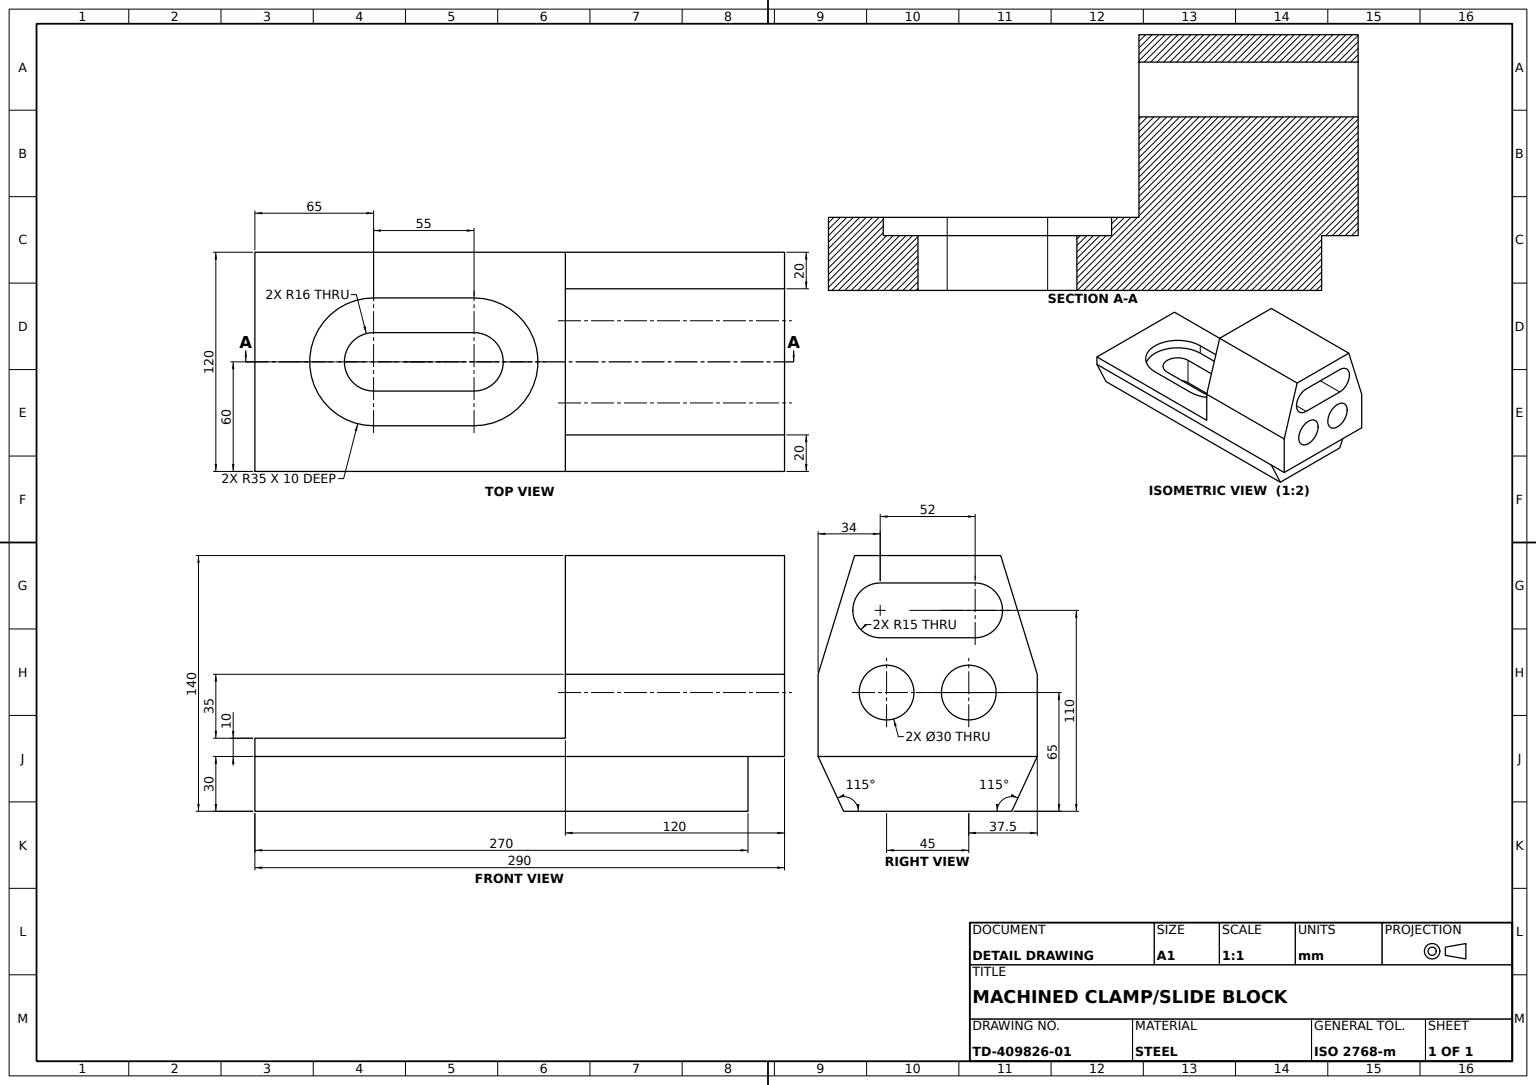
SolidWorks part; units mm, degrees
material "Plain Carbon Steel"
ref_plane "Front Plane" through (0, 0, 0) normal (0, 0, 1) x (1, 0, 0)
ref_plane "Top Plane" through (0, 0, 0) normal (0, 1, 0) x (1, 0, 0)
ref_plane "Right Plane" through (0, 0, 0) normal (1, 0, 0) x (0, 0, -1)
sketch "Base Plate Sketch" plane through (0, 0, 0) normal (0, 1, 0) x (1, 0, 0)
  line L1 (145, 0) -> (145, 60)
  line L2 (145, 60) -> (-145, 60)
  line L3 (-145, 60) -> (-145, -60)
  line L4 (-145, -60) -> (145, -60)
  line L5 (145, -60) -> (145, 0)
  dimension "D1" = 290
  dimension "D2" = 120
  dimension "D3" = 145
  dimension "D4" = 60
  dimension "D5" = 60
extrude "Base Plate" add sketch "Base Plate Sketch" along normal blind 10
sketch "Lower Rail Sketch" plane through (-145, 0, 0) normal (-1, 0, 0) x (0, 0, 1)
  line L2 (60, 0) -> (46.0108, -30)
  line L3 (46.0108, -30) -> (-46.0108, -30)
  line L4 (-60, 0) -> (-46.0108, -30)
  line L5 (-60, 0) -> (60, 0)
  dimension "D1" = 92.0215
  dimension "D2" = 13.9892
  dimension "D3" = 115
  dimension "D4" = 33.1013
extrude "Lower Rail" add sketch "Lower Rail Sketch" against normal blind 270
ref_plane "Upper Block Plane" through (25, 0, 0) normal (1, 0, 0) x (0, 0, -1)
sketch "Upper Block Sketch" plane through (25, 0, 0) normal (1, 0, 0) x (0, 0, -1)
  line L2 (0, 110) -> (40, 110)
  line L3 (0, 110) -> (-40, 110)
  line L4 (60, 10) -> (60, 45)
  line L5 (60, 45) -> (40, 110)
  line L6 (-60, 10) -> (-60, 45)
  line L7 (-60, 45) -> (-40, 110)
  line L8 (-60, 10) -> (60, 10)
  dimension "D1" = 40
  dimension "D2" = 20
  dimension "D3" = 20
  dimension "D4" = 65
  dimension "D5" = 65
  dimension "D6" = 100
extrude "Upper Block" add sketch "Upper Block Sketch" along normal blind 120
sketch "Block Holes and Slot Sketch" plane through (25, 0, 0) normal (-1, 0, 0) x (0, 0, 1)
  line L0 (-26, 95) -> (26, 95)
  line L3 (-26, 65) -> (26, 65)
  circle A0 centre (22.5, 35) radius 15
  circle A1 centre (-22.5, 35) radius 15
  arc A2 (26, 65) -> (26, 95) centre (26, 80) ccw
  arc A3 (-26, 95) -> (-26, 65) centre (-26, 80) ccw
  dimension "D1" = 15
  dimension "D4" = 30
  dimension "D5" = 30
  dimension "D2" = 52
  dimension "D3" = 45
  dimension "D6" = 22.5
  dimension "D7" = 35
  dimension "D8" = 41.6083
  dimension "D9" = 80
  dimension "D10" = 26
extrude "Block Holes and Slot" cut sketch "Block Holes and Slot Sketch" against normal blind 212
sketch "Base Slot Counterbore Sketch" plane through (0, 10, 0) normal (0, 1, 0) x (1, 0, 0)
  line L3 (-80, 35) -> (-25, 35)
  line L4 (-80, -35) -> (-25, -35)
  arc A0 (-25, -35) -> (-25, 35) centre (-25, 0) ccw
  arc A1 (-80, 35) -> (-80, -35) centre (-80, 0) ccw
  dimension "D1" = 35
  dimension "D2" = 80
  dimension "D3" = 25
extrude "Base Slot Counterbore" cut sketch "Base Slot Counterbore Sketch" against normal blind 10
sketch "Base Through Slot Sketch" plane through (0, 0, 0) normal (0, 1, 0) x (1, 0, 0)
  line L0 (-80, 16) -> (-25, 16)
  line L1 (-80, -16) -> (-25, -16)
  arc A0 (-80, 16) -> (-80, -16) centre (-80, 0) ccw
  arc A1 (-25, -16) -> (-25, 16) centre (-25, 0) ccw
  dimension "D1" = 16
extrude "Base Through Slot" cut sketch "Base Through Slot Sketch" against normal blind 68
